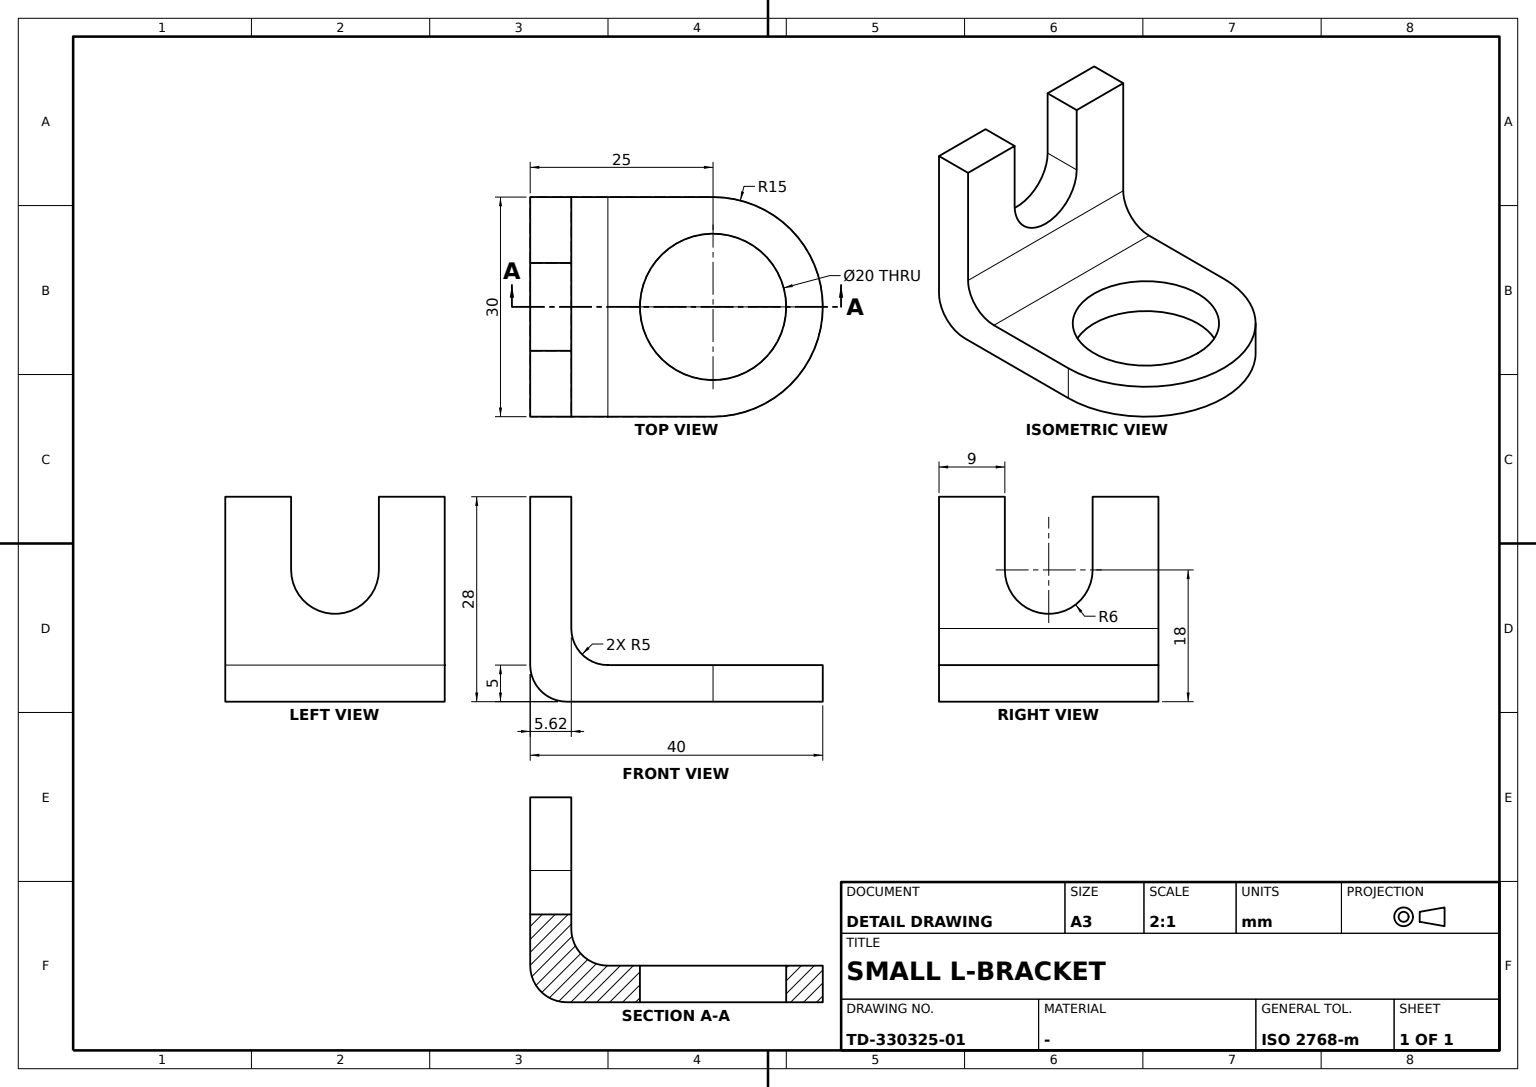
CATIA V5 part; units mm, degrees
sketch "Sketch1" plane through (0, 0, 0) normal (0, 0, 1) x (0, 1, 0)
  arc A0 (-15, 0) -> (15, 0) centre (0, 0) ccw
  point P0 (15, 0)
  line L0 (15, 0) -> (15, 25)
  point P1 (15, 25)
  point P2 (-15, 25)
  point P3 (-15, 0)
  line L1 (-15, 0) -> (-15, 25)
  line L2 (-15, 25) -> (15, 25)
  point P4 (-15, 0)
  point P5 (15, 0)
  dimension "radius A0" = 15
  dimension "length L0" = 25
  constraint coincidence P0 A0
  constraint coincidence P0 x-axis
  constraint coincidence L0 P5
  constraint coincidence L1 P4
  constraint coincidence P0 P5
  constraint coincidence P3 P4
  constraint tangency L0 A0
  constraint symmetry P1 P2 y-axis
  constraint symmetry P0 P3 y-axis
  constraint symmetry L0 L1 y-axis
  constraint horizontal L2 x-axis
extrude "Pad1" add sketch "Sketch1" along normal blind 5
sketch "Sketch2" plane through (0, 0, 5) normal (0, 0, 1) x (0, 1, 0)
  line L0 (-15, 25) -> (15, 25)
  line L1 (15, 25) -> (15, 19.3809)
  line L2 (15, 19.3809) -> (-15, 19.3809)
  line L3 (-15, 19.3809) -> (-15, 25)
  line L4 (15, 25) -> (-15, 25) construction
  line L5 (15, 0) -> (15, 25) construction
  dimension "length L2" = 30
  constraint horizontal L0 x-axis
  constraint horizontal L2 x-axis
  constraint vertical L1 y-axis
  constraint vertical L3 y-axis
  constraint coincidence L0 L4
  constraint coincidence L1 L5
extrude "Pad2" add sketch "Sketch2" along normal blind 23
sketch "Sketch3" plane through (-25, 0, 0) normal (-1, 0, 0) x (0, -1, 0)
  arc A0 (-6, 18) -> (6, 18) centre (0, 18) ccw
  point P0 (0, 18)
  line L0 (-15, 28) -> (15, 28) construction
  point P1 (-6, 18)
  line L1 (-6, 18) -> (-6, 28.291)
  point P2 (-6, 28.291)
  point P3 (6, 28.291)
  point P4 (6, 18)
  line L2 (6, 18) -> (6, 28.291)
  line L3 (-6, 28.291) -> (6, 28.291)
  point P5 (6, 18)
  dimension "radius A0" = 6
  dimension "distance L0 P0" = 10
  constraint coincidence P0 y-axis
  constraint coincidence L2 P5
  constraint coincidence P4 P5
  constraint tangency L1 A0
  constraint horizontal L3 x-axis
extrude "Pocket1" cut sketch "Sketch3" against normal up to next
sketch "Sketch4" plane through (10.6066, -3.2226, 5) normal (0, 0, 1) x (1, 0, 0)
  point P0 (-10.6066, 3.2226)
  arc A0 (-10.6066, -11.7774) -> (-10.6066, 18.2226) centre (-10.6066, 3.2226) ccw construction
  constraint concentricity A0 P0
hole "Hole1" at (0, 0, 5) direction (0, 0, -1) diameter 20 depth 10
fillet "Fillet1" radius 5 1 edges at (-25, 0, 0)
fillet "Fillet2" radius 5 1 edges at (-19.3809, 0, 5)
properties part number "catia 16"
